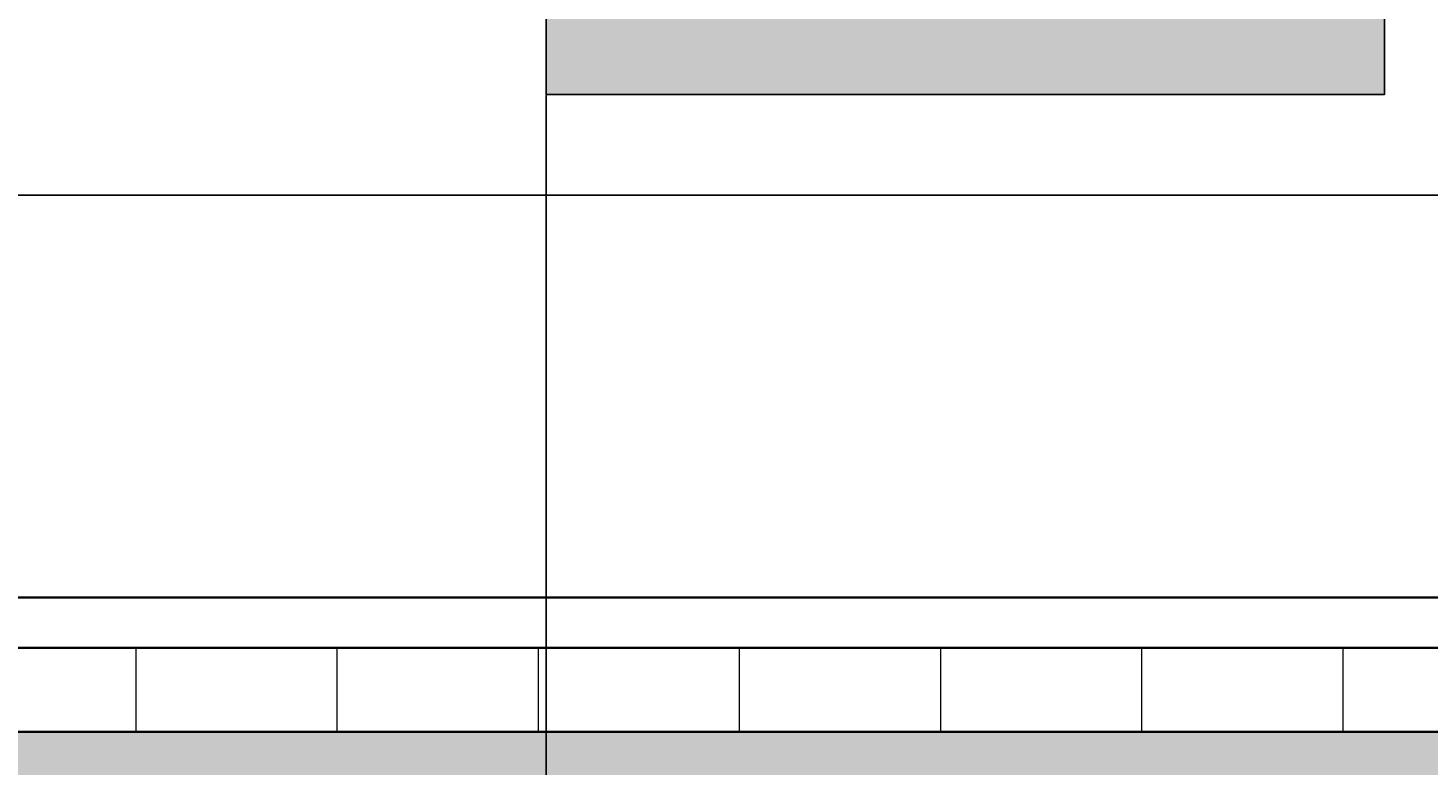
# Model space of a CAD drawing. Units: inches. Extents: x -301 to 715, y -607 to 364.
# Tile 25 of 141: x 18 to 101, y -474 to -430. Entities that reach past the tile are written whole.
import ezdxf

# ---------------------------------------------------------------- set-up
doc = ezdxf.new("R2010")
doc.units = ezdxf.units.IN
doc.header["$MEASUREMENT"] = 0
for name, color, linetype, lineweight in [('A-ANNO-DIMS', 2, 'Continuous', 18), ('A-GLAZ', 2, 'Continuous', 25), ('A-SECT', 1, 'Continuous', 35), ('A-SECT-PATT', 8, 'Continuous', 13)]:
    doc.layers.add(name, color=color, linetype=linetype, lineweight=lineweight)
doc.styles.get("Standard").update_dxf_attribs({"font": 'arial.ttf'})
doc.dimstyles.get("Standard").update_dxf_attribs({"dimtxt": 0.18, "dimasz": 0.18, "dimexe": 0.18, "dimexo": 0.0625, "dimgap": 0.09, "dimtad": 0, "dimtih": 1, "dimtoh": 1, "dimdec": 1, "dimzin": 0, "dimdsep": 46, "dimlunit": 4, "dimtxsty": 'Standard', "dimcen": 0.09, "dimclrd": 3, "dimclre": 4, "dimclrt": 6, "dimadec": 0, "dimazin": 0, "dimtfac": 1, "dimtdec": 1, "dimtofl": 0, "dimtmove": 0, "dimatfit": 3, "dimfxl": 1, "dimtfill": 2, "dimtfillclr": 51, "dimtolj": 1, "dimtzin": 0, "dimarcsym": 0})

# ---------------------------------------------------------------- blocks, each defined once
blk = doc.blocks.new('*D176')
at = {"layer": 'A-ANNO-DIMS', "color": 4, "lineweight": -2, "transparency": 16777216}
for p, q in [((148.28, -324.477), (215.605, -324.477)), ((-15.22, -540.477), (215.605, -540.477))]:
    blk.add_line(p, q, dxfattribs=at)
at = {"layer": 'A-ANNO-DIMS', "color": 3, "lineweight": -2, "transparency": 16777216}
for p, q in [((215.425, -324.657), (215.425, -432.296)), ((215.425, -540.297), (215.425, -432.659))]:
    blk.add_line(p, q, dxfattribs=at)
at = {"layer": 'A-ANNO-DIMS', "color": 3, "transparency": 16777216}
for points in [[(215.395, -324.657), (215.455, -324.657), (215.425, -324.477)], [(215.395, -540.297), (215.455, -540.297), (215.425, -540.477)]]:
    blk.add_solid(points, dxfattribs=at)
at = {"layer": 'Defpoints', "color": 0, "transparency": 16777216}
for p in [(148.218, -324.477), (-15.282, -540.477), (215.425, -540.477)]:
    blk.add_point(p, dxfattribs=at)
at = {"layer": 'A-ANNO-DIMS', "color": 6, "transparency": 16777216, "insert": (215.425, -432.477), "char_height": 0.18, "attachment_point": 5, "bg_fill": 1, "box_fill_scale": 1.25, "bg_fill_color": 51, "bg_fill_transparency": 0}
blk.add_mtext('\\A1;18\'-0"', dxfattribs=at)
blk = doc.blocks.new('*D181')
at = {"layer": 'A-ANNO-DIMS', "color": 4, "lineweight": -2, "transparency": 16777216}
for p, q in [((48.468, -433.54), (48.468, -573.809)), ((12.718, -463.54), (12.718, -573.809))]:
    blk.add_line(p, q, dxfattribs=at)
at = {"layer": 'A-ANNO-DIMS', "color": 3, "lineweight": -2, "transparency": 16777216}
for p, q in [((12.898, -573.629), (30.264, -573.629)), ((48.288, -573.629), (30.922, -573.629))]:
    blk.add_line(p, q, dxfattribs=at)
at = {"layer": 'A-ANNO-DIMS', "color": 3, "transparency": 16777216}
for points in [[(12.898, -573.599), (12.898, -573.659), (12.718, -573.629)], [(48.288, -573.599), (48.288, -573.659), (48.468, -573.629)]]:
    blk.add_solid(points, dxfattribs=at)
at = {"layer": 'Defpoints', "color": 0, "transparency": 16777216}
for p in [(48.468, -433.477), (12.718, -463.477), (48.468, -573.629)]:
    blk.add_point(p, dxfattribs=at)
at = {"layer": 'A-ANNO-DIMS', "color": 6, "transparency": 16777216, "insert": (30.593, -573.629), "char_height": 0.18, "attachment_point": 5, "bg_fill": 1, "box_fill_scale": 1.25, "bg_fill_color": 51, "bg_fill_transparency": 0}
blk.add_mtext('\\A1;3\'-0"', dxfattribs=at)
blk = doc.blocks.new('*D187')
at = {"layer": 'A-ANNO-DIMS', "color": 4, "lineweight": -2, "transparency": 16777216}
for p, q in [((139.674, -385.477), (-266.112, -385.477)), ((143.155, -439.477), (-266.112, -439.477))]:
    blk.add_line(p, q, dxfattribs=at)
at = {"layer": 'A-ANNO-DIMS', "color": 3, "lineweight": -2, "transparency": 16777216}
for p, q in [((-265.932, -385.657), (-265.932, -412.296)), ((-265.932, -439.297), (-265.932, -412.659))]:
    blk.add_line(p, q, dxfattribs=at)
at = {"layer": 'A-ANNO-DIMS', "color": 3, "transparency": 16777216}
for points in [[(-265.962, -385.657), (-265.902, -385.657), (-265.932, -385.477)], [(-265.962, -439.297), (-265.902, -439.297), (-265.932, -439.477)]]:
    blk.add_solid(points, dxfattribs=at)
at = {"layer": 'Defpoints', "color": 0, "transparency": 16777216}
for p in [(-265.932, -385.477), (139.737, -385.477), (143.218, -439.477)]:
    blk.add_point(p, dxfattribs=at)
at = {"layer": 'A-ANNO-DIMS', "color": 6, "transparency": 16777216, "insert": (-265.932, -412.477), "char_height": 0.18, "attachment_point": 5, "bg_fill": 1, "box_fill_scale": 1.25, "bg_fill_color": 51, "bg_fill_transparency": 0}
blk.add_mtext('\\A1;4\'-6"', dxfattribs=at)

msp = doc.modelspace()

# ---------------------------------------------------------------- hatches: boundary and pattern name
at = {"layer": 'A-SECT-PATT'}
h = msp.add_hatch(dxfattribs=at)
h.set_pattern_fill('AR-CONC', color=256, scale=0.5)
h.set_pattern_definition([(50, (10.3213, 33.8764), (3.586301, -0.31376), [0.375, -4.125]), (355, (10.3213, 33.8764), (-0.693757, 3.76096), [0.3, -3.3]), (100.45144, (10.62, 33.8502), (2.892544, 3.4472), [0.3187, -3.50571]), (46.1842, (10.3213, 34.8764), (5.336207, -0.827596), [0.5625, -6.1875]), (96.6356, (10.766, 34.8074), (4.67331, 4.870593), [0.47805, -5.25857]), (351.1842, (10.321, 34.8764), (4.67331, 4.870593), [0.45, -4.95]), (21, (10.8213, 34.6264), (2.984535, -2.013094), [0.375, -4.125]), (326, (10.8213, 34.6264), (1.216577, 3.62575), [0.3, -3.3]), (71.45144, (11.07, 34.4586), (4.201112, 1.612656), [0.3187, -3.50571]), (37.5, (10.3213, 33.8764), (0.0607993, 1.6644693), [0, -3.26, 0, -3.35, 0, -3.3125]), (7.5, (10.3213, 33.8764), (1.3153477, 1.9720586), [0, -1.91, 0, -3.185, 0, -1.2625]), (327.5, (9.2063, 33.8764), (2.6691122, -0.1127744), [0, -1.25, 0, -3.9, 0, -5.175]), (317.5, (8.7063, 33.8764), (2.915931, 0.500525), [0, -1.625, 0, -2.59, 0, -3.675])])
h.paths.add_polyline_path([(-56.282, -535.477), (-61.282, -535.477), (-61.282, -540.477), (-15.282, -540.477), (-15.282, -535.477), (-20.282, -535.477)])
h.paths.add_polyline_path([(119.255, -535.477), (114.255, -535.477), (114.255, -540.477), (163.255, -540.477), (163.255, -535.477), (158.255, -535.477)])
h.paths.add_polyline_path([(-206.282, -471.477), (-209.282, -471.477), (-209.282, -481.477), (-206.282, -481.477), (-194.282, -481.477), (-194.282, -471.477)])
h.paths.add_polyline_path([(-41.282, -481.477), (-41.282, -471.477), (-185.282, -471.477), (-185.282, -481.477), (-180.282, -481.477)])
h.paths.add_polyline_path([(134.255, -481.477), (134.255, -471.477), (-35.282, -471.477), (-35.282, -481.477), (-30.282, -481.477)])
h.paths.add_polyline_path([(155.218, -481.477), (158.218, -481.477), (158.218, -471.477), (153.218, -471.477), (143.218, -471.477), (143.218, -481.477), (148.255, -481.477)])
h.paths.add_polyline_path([(-193.88, -356.477), (-193.904, -361.477), (143.218, -361.477), (143.218, -356.477)])
h = msp.add_hatch(color=256, dxfattribs=at)
h.dxf.hatch_style = 1
h.paths.add_polyline_path([(-138.282, -385.477), (-138.282, -433.477), (-87.981, -433.477), (-87.981, -385.477)])
h.paths.add_polyline_path([(-92.981, -390.477), (-92.981, -428.477), (-133.282, -428.477), (-133.282, -390.477)], flags=16)
h.paths.add_polyline_path([(-35.282, -385.477), (-35.282, -463.477), (12.718, -463.477), (12.718, -385.477)])
h.paths.add_polyline_path([(-30.282, -390.477), (7.718, -390.477), (7.718, -458.477), (-30.282, -458.477)], flags=16)
h.paths.add_polyline_path([(48.468, -385.477), (48.468, -433.477), (98.468, -433.477), (98.468, -385.477)])
h.paths.add_polyline_path([(93.468, -390.477), (93.468, -428.477), (53.468, -428.477), (53.468, -390.477)], flags=16)
h = msp.add_hatch(dxfattribs=at)
h.set_pattern_fill('ANSI31', color=256, scale=96, angle=45, style=0)
h.paths.add_polyline_path([(-35.282, -471.477), (134.255, -471.477), (134.255, -466.477), (-35.282, -466.477)])

# ---------------------------------------------------------------- linework, layer by layer
at = {"layer": 'A-GLAZ'}
msp.add_lwpolyline([(48.468, -385.477), (98.468, -385.477), (98.468, -433.477), (48.468, -433.477)], close=True, dxfattribs=at)
at = {"layer": 'A-SECT'}
for p, q in [((-199.282, -463.477), (148.255, -463.477)), ((-204.282, -466.477), (153.218, -466.477)), ((-206.282, -471.477), (155.218, -471.477))]:
    msp.add_line(p, q, dxfattribs=at)

# ---------------------------------------------------------------- dimensions: what is measured, and where the dimension line sits
at = {"layer": 'A-ANNO-DIMS'}
for base, p1, p2, picture, middle in [((215.425, -540.477), (148.218, -324.477), (-15.282, -540.477), '*D176', (215.425, -432.477)), ((-265.932, -385.477), (143.218, -439.477), (139.737, -385.477), '*D187', (-265.932, -412.477))]:
    dim = msp.add_linear_dim(base=base, p1=p1, p2=p2, angle=90, dimstyle='Standard', override={"dimdec": 1, "dimlfac": 1, "dimrnd": 0, "dimzin": 1, "dimdsep": 46, "dimlunit": 4, "dimfrac": 2}, dxfattribs=at)
    dim.commit()
    dim.dimension.update_dxf_attribs({"geometry": picture, "text_midpoint": middle})
dim = msp.add_linear_dim(base=(48.467984, -573.628877), p1=(12.717984, -463.47741), p2=(48.467984, -433.47741), dimstyle='Standard', override={"dimdec": 1, "dimlfac": 1, "dimrnd": 0, "dimzin": 1, "dimdsep": 46, "dimlunit": 4, "dimfrac": 2}, dxfattribs=at)
dim.commit()
dim.dimension.update_dxf_attribs({"geometry": '*D181', "text_midpoint": (30.592984, -573.628877)})

doc.saveas('drawing.dxf')
